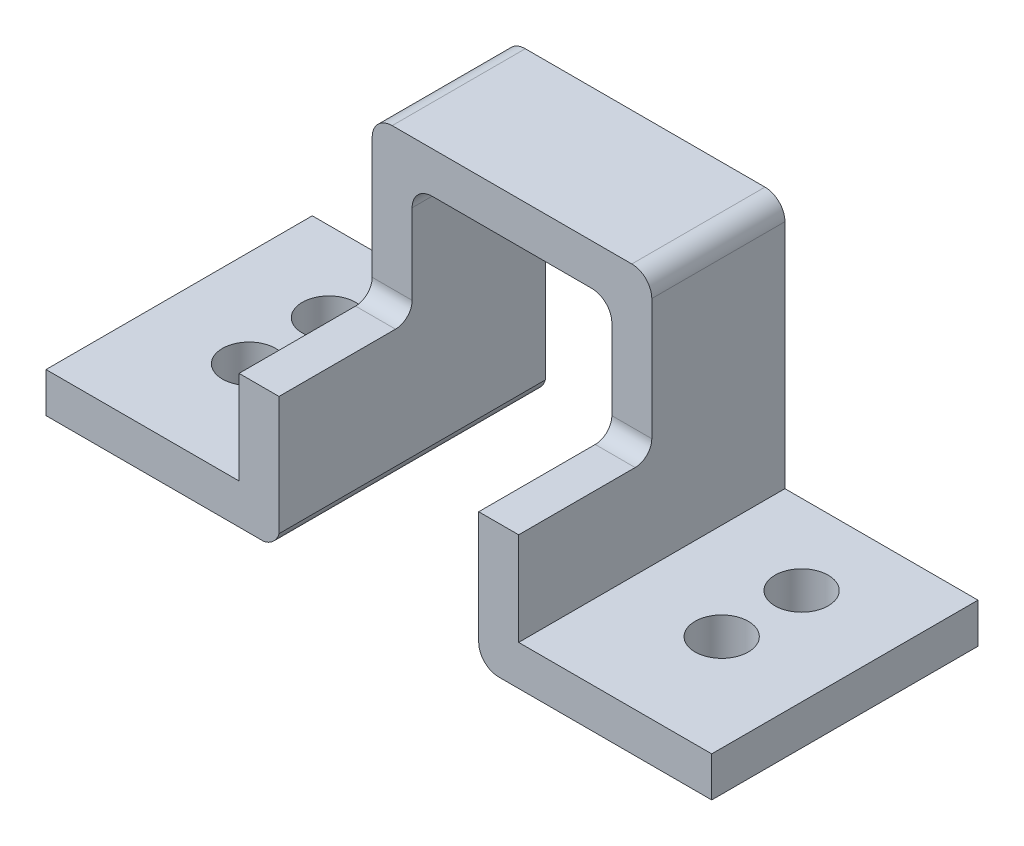
ISO-10303-21;
HEADER;
FILE_DESCRIPTION(('STEP AP214'),'2;1');
FILE_NAME('part.step','',(''),(''),'','','');
FILE_SCHEMA(('AUTOMOTIVE_DESIGN { 1 0 10303 214 1 1 1 1 }'));
ENDSEC;
DATA;
#1=APPLICATION_CONTEXT('core data for automotive mechanical design processes');
#2=APPLICATION_PROTOCOL_DEFINITION('international standard','automotive_design',2000,#1);
#3=PRODUCT_CONTEXT('',#1,'mechanical');
#4=PRODUCT('Part','Part','',(#3));
#5=PRODUCT_RELATED_PRODUCT_CATEGORY('part','',(#4));
#6=PRODUCT_DEFINITION_FORMATION('','',#4);
#7=PRODUCT_DEFINITION_CONTEXT('part definition',#1,'design');
#8=PRODUCT_DEFINITION('design','',#6,#7);
#9=PRODUCT_DEFINITION_SHAPE('','',#8);
#10=(LENGTH_UNIT() NAMED_UNIT(*) SI_UNIT(.MILLI.,.METRE.));
#11=(NAMED_UNIT(*) PLANE_ANGLE_UNIT() SI_UNIT($,.RADIAN.));
#12=(NAMED_UNIT(*) SI_UNIT($,.STERADIAN.) SOLID_ANGLE_UNIT());
#13=UNCERTAINTY_MEASURE_WITH_UNIT(LENGTH_MEASURE(1.E-05),#10,'distance_accuracy_value','');
#14=(GEOMETRIC_REPRESENTATION_CONTEXT(3) GLOBAL_UNCERTAINTY_ASSIGNED_CONTEXT((#13)) GLOBAL_UNIT_ASSIGNED_CONTEXT((#10,
#11,#12)) REPRESENTATION_CONTEXT('',''));
#15=CARTESIAN_POINT('',(0.,0.,0.));
#16=DIRECTION('',(0.,0.,1.));
#17=DIRECTION('',(1.,0.,0.));
#18=AXIS2_PLACEMENT_3D('',#15,#16,#17);
#19=CARTESIAN_POINT('',(0.,20.,28.));
#20=DIRECTION('',(0.,1.,0.));
#21=DIRECTION('',(0.,0.,1.));
#22=AXIS2_PLACEMENT_3D('',#19,#20,#21);
#23=PLANE('',#22);
#24=DIRECTION('',(0.,0.,-1.));
#25=VECTOR('',#24,1.);
#26=CARTESIAN_POINT('',(36.,20.,28.));
#27=LINE('',#26,#25);
#28=CARTESIAN_POINT('',(36.,20.,20.));
#29=VERTEX_POINT('',#28);
#30=CARTESIAN_POINT('',(36.,20.,2.49999999999997));
#31=VERTEX_POINT('',#30);
#32=EDGE_CURVE('E359',#29,#31,#27,.T.);
#33=ORIENTED_EDGE('',*,*,#32,.T.);
#34=DIRECTION('',(1.,0.,0.));
#35=VECTOR('',#34,1.);
#36=CARTESIAN_POINT('',(30.,20.,2.49999999999998));
#37=LINE('',#36,#35);
#38=CARTESIAN_POINT('',(30.,20.,2.49999999999997));
#39=VERTEX_POINT('',#38);
#40=EDGE_CURVE('E394',#39,#31,#37,.T.);
#41=ORIENTED_EDGE('',*,*,#40,.F.);
#42=DIRECTION('',(0.,0.,-1.));
#43=VECTOR('',#42,1.);
#44=CARTESIAN_POINT('',(30.,20.,28.));
#45=LINE('',#44,#43);
#46=CARTESIAN_POINT('',(30.,20.,20.));
#47=VERTEX_POINT('',#46);
#48=EDGE_CURVE('E323',#47,#39,#45,.T.);
#49=ORIENTED_EDGE('',*,*,#48,.F.);
#50=DIRECTION('',(-1.,0.,0.));
#51=VECTOR('',#50,1.);
#52=CARTESIAN_POINT('',(3.,20.,20.));
#53=LINE('',#52,#51);
#54=EDGE_CURVE('E50',#29,#47,#53,.T.);
#55=ORIENTED_EDGE('',*,*,#54,.F.);
#56=EDGE_LOOP('',(#33,#41,#49,#55));
#57=FACE_BOUND('',#56,.T.);
#58=ADVANCED_FACE('F39',(#57),#23,.T.);
#59=CARTESIAN_POINT('',(0.,0.,0.));
#60=DIRECTION('',(0.,0.,1.));
#61=DIRECTION('',(1.,0.,0.));
#62=AXIS2_PLACEMENT_3D('',#59,#60,#61);
#63=PLANE('',#62);
#64=DIRECTION('',(1.,0.,0.));
#65=VECTOR('',#64,1.);
#66=CARTESIAN_POINT('',(30.,22.5,0.));
#67=LINE('',#66,#65);
#68=CARTESIAN_POINT('',(30.,22.5,0.));
#69=VERTEX_POINT('',#68);
#70=CARTESIAN_POINT('',(36.,22.5,0.));
#71=VERTEX_POINT('',#70);
#72=EDGE_CURVE('E59',#69,#71,#67,.T.);
#73=ORIENTED_EDGE('',*,*,#72,.T.);
#74=DIRECTION('',(0.,1.,0.));
#75=VECTOR('',#74,1.);
#76=CARTESIAN_POINT('',(36.,0.,0.));
#77=LINE('',#76,#75);
#78=CARTESIAN_POINT('',(36.,40.7317104418747,0.));
#79=VERTEX_POINT('',#78);
#80=EDGE_CURVE('E358',#71,#79,#77,.T.);
#81=ORIENTED_EDGE('',*,*,#80,.T.);
#82=CARTESIAN_POINT('',(33.,40.7317104418747,0.));
#83=DIRECTION('',(0.,0.,1.));
#84=DIRECTION('',(1.,0.,0.));
#85=AXIS2_PLACEMENT_3D('',#82,#83,#84);
#86=CIRCLE('',#85,3.);
#87=CARTESIAN_POINT('',(33.,43.7317104418747,0.));
#88=VERTEX_POINT('',#87);
#89=EDGE_CURVE('E356',#79,#88,#86,.T.);
#90=ORIENTED_EDGE('',*,*,#89,.T.);
#91=DIRECTION('',(-1.,0.,0.));
#92=VECTOR('',#91,1.);
#93=CARTESIAN_POINT('',(0.,43.7317104418747,0.));
#94=LINE('',#93,#92);
#95=CARTESIAN_POINT('',(-3.,43.7317104418747,0.));
#96=VERTEX_POINT('',#95);
#97=EDGE_CURVE('E339',#88,#96,#94,.T.);
#98=ORIENTED_EDGE('',*,*,#97,.T.);
#99=CARTESIAN_POINT('',(-3.,40.7317104418747,0.));
#100=DIRECTION('',(0.,0.,1.));
#101=DIRECTION('',(1.,0.,0.));
#102=AXIS2_PLACEMENT_3D('',#99,#100,#101);
#103=CIRCLE('',#102,3.);
#104=CARTESIAN_POINT('',(-6.,40.7317104418747,0.));
#105=VERTEX_POINT('',#104);
#106=EDGE_CURVE('E344',#96,#105,#103,.T.);
#107=ORIENTED_EDGE('',*,*,#106,.T.);
#108=DIRECTION('',(0.,-1.,0.));
#109=VECTOR('',#108,1.);
#110=CARTESIAN_POINT('',(-5.99999999999999,0.,0.));
#111=LINE('',#110,#109);
#112=CARTESIAN_POINT('',(-6.,22.5,0.));
#113=VERTEX_POINT('',#112);
#114=EDGE_CURVE('E343',#105,#113,#111,.T.);
#115=ORIENTED_EDGE('',*,*,#114,.T.);
#116=DIRECTION('',(-1.,0.,0.));
#117=VECTOR('',#116,1.);
#118=CARTESIAN_POINT('',(0.,22.5,0.));
#119=LINE('',#118,#117);
#120=CARTESIAN_POINT('',(0.,22.5,0.));
#121=VERTEX_POINT('',#120);
#122=EDGE_CURVE('E219',#121,#113,#119,.T.);
#123=ORIENTED_EDGE('',*,*,#122,.F.);
#124=DIRECTION('',(0.,1.,0.));
#125=VECTOR('',#124,1.);
#126=CARTESIAN_POINT('',(0.,0.,0.));
#127=LINE('',#126,#125);
#128=CARTESIAN_POINT('',(0.,34.547795072297,0.));
#129=VERTEX_POINT('',#128);
#130=EDGE_CURVE('E349',#121,#129,#127,.T.);
#131=ORIENTED_EDGE('',*,*,#130,.T.);
#132=CARTESIAN_POINT('',(3.,34.547795072297,0.));
#133=DIRECTION('',(0.,0.,1.));
#134=DIRECTION('',(1.,0.,0.));
#135=AXIS2_PLACEMENT_3D('',#132,#133,#134);
#136=CIRCLE('',#135,3.);
#137=CARTESIAN_POINT('',(3.,37.547795072297,0.));
#138=VERTEX_POINT('',#137);
#139=EDGE_CURVE('E346',#129,#138,#136,.F.);
#140=ORIENTED_EDGE('',*,*,#139,.T.);
#141=DIRECTION('',(1.,0.,0.));
#142=VECTOR('',#141,1.);
#143=CARTESIAN_POINT('',(0.,37.547795072297,0.));
#144=LINE('',#143,#142);
#145=CARTESIAN_POINT('',(27.,37.547795072297,0.));
#146=VERTEX_POINT('',#145);
#147=EDGE_CURVE('E353',#138,#146,#144,.T.);
#148=ORIENTED_EDGE('',*,*,#147,.T.);
#149=CARTESIAN_POINT('',(27.,34.547795072297,0.));
#150=DIRECTION('',(0.,0.,1.));
#151=DIRECTION('',(1.,0.,0.));
#152=AXIS2_PLACEMENT_3D('',#149,#150,#151);
#153=CIRCLE('',#152,3.);
#154=CARTESIAN_POINT('',(30.,34.547795072297,0.));
#155=VERTEX_POINT('',#154);
#156=EDGE_CURVE('E351',#146,#155,#153,.F.);
#157=ORIENTED_EDGE('',*,*,#156,.T.);
#158=DIRECTION('',(0.,-1.,0.));
#159=VECTOR('',#158,1.);
#160=CARTESIAN_POINT('',(30.,0.,0.));
#161=LINE('',#160,#159);
#162=EDGE_CURVE('E53',#155,#69,#161,.T.);
#163=ORIENTED_EDGE('',*,*,#162,.T.);
#164=EDGE_LOOP('',(#73,#81,#90,#98,#107,#115,#123,#131,#140,#148,#157,#163));
#165=FACE_BOUND('',#164,.T.);
#166=ADVANCED_FACE('F426',(#165),#63,.T.);
#167=CARTESIAN_POINT('',(30.,34.547795072297,20.));
#168=DIRECTION('',(1.,0.,0.));
#169=DIRECTION('',(0.,1.,0.));
#170=AXIS2_PLACEMENT_3D('',#167,#168,#169);
#171=PLANE('',#170);
#172=CARTESIAN_POINT('',(30.,22.5,2.49999999999998));
#173=DIRECTION('',(-1.,0.,0.));
#174=DIRECTION('',(0.,0.,-1.));
#175=AXIS2_PLACEMENT_3D('',#172,#173,#174);
#176=CIRCLE('',#175,2.49999999999997);
#177=EDGE_CURVE('E440',#69,#39,#176,.T.);
#178=ORIENTED_EDGE('',*,*,#177,.F.);
#179=ORIENTED_EDGE('',*,*,#162,.F.);
#180=DIRECTION('',(0.,0.,-1.));
#181=VECTOR('',#180,1.);
#182=CARTESIAN_POINT('',(30.,34.547795072297,20.));
#183=LINE('',#182,#181);
#184=CARTESIAN_POINT('',(30.,34.547795072297,-20.));
#185=VERTEX_POINT('',#184);
#186=EDGE_CURVE('E309',#155,#185,#183,.T.);
#187=ORIENTED_EDGE('',*,*,#186,.T.);
#188=DIRECTION('',(0.,-1.,0.));
#189=VECTOR('',#188,1.);
#190=CARTESIAN_POINT('',(30.,34.547795072297,-20.));
#191=LINE('',#190,#189);
#192=CARTESIAN_POINT('',(30.,3.,-20.));
#193=VERTEX_POINT('',#192);
#194=EDGE_CURVE('E260',#185,#193,#191,.T.);
#195=ORIENTED_EDGE('',*,*,#194,.T.);
#196=DIRECTION('',(0.,0.,1.));
#197=VECTOR('',#196,1.);
#198=CARTESIAN_POINT('',(30.,3.,-20.));
#199=LINE('',#198,#197);
#200=CARTESIAN_POINT('',(30.,3.,20.));
#201=VERTEX_POINT('',#200);
#202=EDGE_CURVE('E210',#193,#201,#199,.T.);
#203=ORIENTED_EDGE('',*,*,#202,.T.);
#204=DIRECTION('',(0.,-1.,0.));
#205=VECTOR('',#204,1.);
#206=CARTESIAN_POINT('',(30.,34.547795072297,20.));
#207=LINE('',#206,#205);
#208=EDGE_CURVE('E217',#47,#201,#207,.T.);
#209=ORIENTED_EDGE('',*,*,#208,.F.);
#210=ORIENTED_EDGE('',*,*,#48,.T.);
#211=EDGE_LOOP('',(#178,#179,#187,#195,#203,#209,#210));
#212=FACE_BOUND('',#211,.T.);
#213=ADVANCED_FACE('F321',(#212),#171,.F.);
#214=CARTESIAN_POINT('',(3.,34.547795072297,20.));
#215=DIRECTION('',(0.,0.,1.));
#216=DIRECTION('',(1.,0.,0.));
#217=AXIS2_PLACEMENT_3D('',#214,#215,#216);
#218=PLANE('',#217);
#219=CARTESIAN_POINT('',(33.,3.,20.));
#220=DIRECTION('',(0.,0.,-1.));
#221=DIRECTION('',(1.,0.,0.));
#222=AXIS2_PLACEMENT_3D('',#219,#220,#221);
#223=CIRCLE('',#222,3.);
#224=CARTESIAN_POINT('',(33.,0.,20.));
#225=VERTEX_POINT('',#224);
#226=EDGE_CURVE('E198',#225,#201,#223,.T.);
#227=ORIENTED_EDGE('',*,*,#226,.F.);
#228=DIRECTION('',(1.,0.,0.));
#229=VECTOR('',#228,1.);
#230=CARTESIAN_POINT('',(30.,0.,20.));
#231=LINE('',#230,#229);
#232=CARTESIAN_POINT('',(65.,0.,20.));
#233=VERTEX_POINT('',#232);
#234=EDGE_CURVE('E215',#225,#233,#231,.T.);
#235=ORIENTED_EDGE('',*,*,#234,.T.);
#236=DIRECTION('',(0.,1.,0.));
#237=VECTOR('',#236,1.);
#238=CARTESIAN_POINT('',(65.,0.,20.));
#239=LINE('',#238,#237);
#240=CARTESIAN_POINT('',(65.,6.,20.));
#241=VERTEX_POINT('',#240);
#242=EDGE_CURVE('E221',#233,#241,#239,.T.);
#243=ORIENTED_EDGE('',*,*,#242,.T.);
#244=DIRECTION('',(-1.,0.,0.));
#245=VECTOR('',#244,1.);
#246=CARTESIAN_POINT('',(65.,6.,20.));
#247=LINE('',#246,#245);
#248=CARTESIAN_POINT('',(36.,6.,20.));
#249=VERTEX_POINT('',#248);
#250=EDGE_CURVE('E222',#241,#249,#247,.T.);
#251=ORIENTED_EDGE('',*,*,#250,.T.);
#252=DIRECTION('',(0.,1.,0.));
#253=VECTOR('',#252,1.);
#254=CARTESIAN_POINT('',(36.,6.,20.));
#255=LINE('',#254,#253);
#256=EDGE_CURVE('E235',#249,#29,#255,.T.);
#257=ORIENTED_EDGE('',*,*,#256,.T.);
#258=ORIENTED_EDGE('',*,*,#54,.T.);
#259=ORIENTED_EDGE('',*,*,#208,.T.);
#260=EDGE_LOOP('',(#227,#235,#243,#251,#257,#258,#259));
#261=FACE_BOUND('',#260,.T.);
#262=ADVANCED_FACE('F212',(#261),#218,.T.);
#263=CARTESIAN_POINT('',(3.,34.547795072297,-20.));
#264=DIRECTION('',(0.,0.,1.));
#265=DIRECTION('',(1.,0.,0.));
#266=AXIS2_PLACEMENT_3D('',#263,#264,#265);
#267=PLANE('',#266);
#268=DIRECTION('',(1.,0.,0.));
#269=VECTOR('',#268,1.);
#270=CARTESIAN_POINT('',(30.,0.,-20.));
#271=LINE('',#270,#269);
#272=CARTESIAN_POINT('',(33.,0.,-20.));
#273=VERTEX_POINT('',#272);
#274=CARTESIAN_POINT('',(65.,0.,-20.));
#275=VERTEX_POINT('',#274);
#276=EDGE_CURVE('E258',#273,#275,#271,.T.);
#277=ORIENTED_EDGE('',*,*,#276,.F.);
#278=CARTESIAN_POINT('',(33.,3.,-20.));
#279=DIRECTION('',(0.,0.,-1.));
#280=DIRECTION('',(1.,0.,0.));
#281=AXIS2_PLACEMENT_3D('',#278,#279,#280);
#282=CIRCLE('',#281,3.);
#283=EDGE_CURVE('E201',#273,#193,#282,.T.);
#284=ORIENTED_EDGE('',*,*,#283,.T.);
#285=ORIENTED_EDGE('',*,*,#194,.F.);
#286=CARTESIAN_POINT('',(27.,34.547795072297,-20.));
#287=DIRECTION('',(0.,0.,-1.));
#288=DIRECTION('',(1.,0.,0.));
#289=AXIS2_PLACEMENT_3D('',#286,#287,#288);
#290=CIRCLE('',#289,3.);
#291=CARTESIAN_POINT('',(27.,37.547795072297,-20.));
#292=VERTEX_POINT('',#291);
#293=EDGE_CURVE('E251',#292,#185,#290,.T.);
#294=ORIENTED_EDGE('',*,*,#293,.F.);
#295=DIRECTION('',(1.,0.,0.));
#296=VECTOR('',#295,1.);
#297=CARTESIAN_POINT('',(3.,37.547795072297,-20.));
#298=LINE('',#297,#296);
#299=CARTESIAN_POINT('',(3.,37.547795072297,-20.));
#300=VERTEX_POINT('',#299);
#301=EDGE_CURVE('E252',#300,#292,#298,.T.);
#302=ORIENTED_EDGE('',*,*,#301,.F.);
#303=CARTESIAN_POINT('',(3.,34.547795072297,-20.));
#304=DIRECTION('',(0.,0.,-1.));
#305=DIRECTION('',(1.,0.,0.));
#306=AXIS2_PLACEMENT_3D('',#303,#304,#305);
#307=CIRCLE('',#306,3.);
#308=CARTESIAN_POINT('',(0.,34.547795072297,-20.));
#309=VERTEX_POINT('',#308);
#310=EDGE_CURVE('E250',#309,#300,#307,.T.);
#311=ORIENTED_EDGE('',*,*,#310,.F.);
#312=DIRECTION('',(0.,1.,0.));
#313=VECTOR('',#312,1.);
#314=CARTESIAN_POINT('',(0.,0.,-20.));
#315=LINE('',#314,#313);
#316=CARTESIAN_POINT('',(0.,2.14044011670868,-20.));
#317=VERTEX_POINT('',#316);
#318=EDGE_CURVE('E244',#317,#309,#315,.T.);
#319=ORIENTED_EDGE('',*,*,#318,.F.);
#320=CARTESIAN_POINT('',(-2.89404902944698,2.93068072257311,-20.));
#321=DIRECTION('',(0.,0.,-1.));
#322=DIRECTION('',(-1.,0.,0.));
#323=AXIS2_PLACEMENT_3D('',#320,#321,#322);
#324=CIRCLE('',#323,3.);
#325=CARTESIAN_POINT('',(-2.25287003545363,0.,-20.));
#326=VERTEX_POINT('',#325);
#327=EDGE_CURVE('E328',#317,#326,#324,.T.);
#328=ORIENTED_EDGE('',*,*,#327,.T.);
#329=DIRECTION('',(1.,0.,0.));
#330=VECTOR('',#329,1.);
#331=CARTESIAN_POINT('',(-35.,0.,-20.));
#332=LINE('',#331,#330);
#333=CARTESIAN_POINT('',(-35.,0.,-20.));
#334=VERTEX_POINT('',#333);
#335=EDGE_CURVE('E281',#334,#326,#332,.T.);
#336=ORIENTED_EDGE('',*,*,#335,.F.);
#337=DIRECTION('',(0.,-1.,0.));
#338=VECTOR('',#337,1.);
#339=CARTESIAN_POINT('',(-35.,6.,-20.));
#340=LINE('',#339,#338);
#341=CARTESIAN_POINT('',(-35.,6.,-20.));
#342=VERTEX_POINT('',#341);
#343=EDGE_CURVE('E284',#342,#334,#340,.T.);
#344=ORIENTED_EDGE('',*,*,#343,.F.);
#345=DIRECTION('',(-1.,0.,0.));
#346=VECTOR('',#345,1.);
#347=CARTESIAN_POINT('',(-6.,6.,-20.));
#348=LINE('',#347,#346);
#349=CARTESIAN_POINT('',(-6.,6.,-20.));
#350=VERTEX_POINT('',#349);
#351=EDGE_CURVE('E278',#350,#342,#348,.T.);
#352=ORIENTED_EDGE('',*,*,#351,.F.);
#353=DIRECTION('',(0.,-1.,0.));
#354=VECTOR('',#353,1.);
#355=CARTESIAN_POINT('',(-6.,40.7317104418747,-20.));
#356=LINE('',#355,#354);
#357=CARTESIAN_POINT('',(-6.,40.7317104418747,-20.));
#358=VERTEX_POINT('',#357);
#359=EDGE_CURVE('E279',#358,#350,#356,.T.);
#360=ORIENTED_EDGE('',*,*,#359,.F.);
#361=CARTESIAN_POINT('',(-3.,40.7317104418747,-20.));
#362=DIRECTION('',(0.,0.,1.));
#363=DIRECTION('',(1.,0.,0.));
#364=AXIS2_PLACEMENT_3D('',#361,#362,#363);
#365=CIRCLE('',#364,3.);
#366=CARTESIAN_POINT('',(-3.,43.7317104418747,-20.));
#367=VERTEX_POINT('',#366);
#368=EDGE_CURVE('E273',#367,#358,#365,.T.);
#369=ORIENTED_EDGE('',*,*,#368,.F.);
#370=DIRECTION('',(-1.,0.,0.));
#371=VECTOR('',#370,1.);
#372=CARTESIAN_POINT('',(33.,43.7317104418747,-20.));
#373=LINE('',#372,#371);
#374=CARTESIAN_POINT('',(33.,43.7317104418747,-20.));
#375=VERTEX_POINT('',#374);
#376=EDGE_CURVE('E275',#375,#367,#373,.T.);
#377=ORIENTED_EDGE('',*,*,#376,.F.);
#378=CARTESIAN_POINT('',(33.,40.7317104418747,-20.));
#379=DIRECTION('',(0.,0.,1.));
#380=DIRECTION('',(1.,0.,0.));
#381=AXIS2_PLACEMENT_3D('',#378,#379,#380);
#382=CIRCLE('',#381,3.);
#383=CARTESIAN_POINT('',(36.,40.7317104418747,-20.));
#384=VERTEX_POINT('',#383);
#385=EDGE_CURVE('E269',#384,#375,#382,.T.);
#386=ORIENTED_EDGE('',*,*,#385,.F.);
#387=DIRECTION('',(0.,1.,0.));
#388=VECTOR('',#387,1.);
#389=CARTESIAN_POINT('',(36.,6.,-20.));
#390=LINE('',#389,#388);
#391=CARTESIAN_POINT('',(36.,6.,-20.));
#392=VERTEX_POINT('',#391);
#393=EDGE_CURVE('E268',#392,#384,#390,.T.);
#394=ORIENTED_EDGE('',*,*,#393,.F.);
#395=DIRECTION('',(-1.,0.,0.));
#396=VECTOR('',#395,1.);
#397=CARTESIAN_POINT('',(65.,6.,-20.));
#398=LINE('',#397,#396);
#399=CARTESIAN_POINT('',(65.,6.,-20.));
#400=VERTEX_POINT('',#399);
#401=EDGE_CURVE('E261',#400,#392,#398,.T.);
#402=ORIENTED_EDGE('',*,*,#401,.F.);
#403=DIRECTION('',(0.,1.,0.));
#404=VECTOR('',#403,1.);
#405=CARTESIAN_POINT('',(65.,0.,-20.));
#406=LINE('',#405,#404);
#407=EDGE_CURVE('E264',#275,#400,#406,.T.);
#408=ORIENTED_EDGE('',*,*,#407,.F.);
#409=EDGE_LOOP('',(#277,#284,#285,#294,#302,#311,#319,#328,#336,#344,#352,#360,#369,#377,#386,
#394,#402,#408));
#410=FACE_BOUND('',#409,.T.);
#411=ADVANCED_FACE('F417',(#410),#267,.F.);
#412=CARTESIAN_POINT('',(0.,0.,20.));
#413=DIRECTION('',(-1.,0.,0.));
#414=DIRECTION('',(0.,0.,1.));
#415=AXIS2_PLACEMENT_3D('',#412,#413,#414);
#416=PLANE('',#415);
#417=CARTESIAN_POINT('',(0.,22.5,2.5));
#418=DIRECTION('',(1.,0.,0.));
#419=DIRECTION('',(0.,-1.,0.));
#420=AXIS2_PLACEMENT_3D('',#417,#418,#419);
#421=CIRCLE('',#420,2.5);
#422=CARTESIAN_POINT('',(0.,20.,2.5));
#423=VERTEX_POINT('',#422);
#424=EDGE_CURVE('E382',#423,#121,#421,.T.);
#425=ORIENTED_EDGE('',*,*,#424,.F.);
#426=DIRECTION('',(0.,0.,-1.));
#427=VECTOR('',#426,1.);
#428=CARTESIAN_POINT('',(0.,20.,28.));
#429=LINE('',#428,#427);
#430=CARTESIAN_POINT('',(0.,20.,20.));
#431=VERTEX_POINT('',#430);
#432=EDGE_CURVE('E361',#431,#423,#429,.T.);
#433=ORIENTED_EDGE('',*,*,#432,.F.);
#434=DIRECTION('',(0.,1.,0.));
#435=VECTOR('',#434,1.);
#436=CARTESIAN_POINT('',(0.,0.,20.));
#437=LINE('',#436,#435);
#438=CARTESIAN_POINT('',(0.,2.14044011670868,20.));
#439=VERTEX_POINT('',#438);
#440=EDGE_CURVE('E227',#439,#431,#437,.T.);
#441=ORIENTED_EDGE('',*,*,#440,.F.);
#442=DIRECTION('',(0.,0.,1.));
#443=VECTOR('',#442,1.);
#444=CARTESIAN_POINT('',(0.,2.14044011670868,-20.));
#445=LINE('',#444,#443);
#446=EDGE_CURVE('E340',#317,#439,#445,.T.);
#447=ORIENTED_EDGE('',*,*,#446,.F.);
#448=ORIENTED_EDGE('',*,*,#318,.T.);
#449=DIRECTION('',(0.,0.,-1.));
#450=VECTOR('',#449,1.);
#451=CARTESIAN_POINT('',(0.,34.547795072297,20.));
#452=LINE('',#451,#450);
#453=EDGE_CURVE('E317',#129,#309,#452,.T.);
#454=ORIENTED_EDGE('',*,*,#453,.F.);
#455=ORIENTED_EDGE('',*,*,#130,.F.);
#456=EDGE_LOOP('',(#425,#433,#441,#447,#448,#454,#455));
#457=FACE_BOUND('',#456,.T.);
#458=ADVANCED_FACE('F41',(#457),#416,.F.);
#459=CARTESIAN_POINT('',(3.,34.547795072297,20.));
#460=DIRECTION('',(0.,0.,-1.));
#461=DIRECTION('',(-1.,0.,0.));
#462=AXIS2_PLACEMENT_3D('',#459,#460,#461);
#463=CYLINDRICAL_SURFACE('',#462,3.);
#464=ORIENTED_EDGE('',*,*,#139,.F.);
#465=ORIENTED_EDGE('',*,*,#453,.T.);
#466=ORIENTED_EDGE('',*,*,#310,.T.);
#467=DIRECTION('',(0.,0.,-1.));
#468=VECTOR('',#467,1.);
#469=CARTESIAN_POINT('',(3.,37.547795072297,20.));
#470=LINE('',#469,#468);
#471=EDGE_CURVE('E313',#138,#300,#470,.T.);
#472=ORIENTED_EDGE('',*,*,#471,.F.);
#473=EDGE_LOOP('',(#464,#465,#466,#472));
#474=FACE_BOUND('',#473,.T.);
#475=ADVANCED_FACE('F424',(#474),#463,.F.);
#476=CARTESIAN_POINT('',(3.,37.547795072297,20.));
#477=DIRECTION('',(0.,1.,0.));
#478=DIRECTION('',(0.,0.,1.));
#479=AXIS2_PLACEMENT_3D('',#476,#477,#478);
#480=PLANE('',#479);
#481=ORIENTED_EDGE('',*,*,#147,.F.);
#482=ORIENTED_EDGE('',*,*,#471,.T.);
#483=ORIENTED_EDGE('',*,*,#301,.T.);
#484=DIRECTION('',(0.,0.,-1.));
#485=VECTOR('',#484,1.);
#486=CARTESIAN_POINT('',(27.,37.547795072297,20.));
#487=LINE('',#486,#485);
#488=EDGE_CURVE('E315',#146,#292,#487,.T.);
#489=ORIENTED_EDGE('',*,*,#488,.F.);
#490=EDGE_LOOP('',(#481,#482,#483,#489));
#491=FACE_BOUND('',#490,.T.);
#492=ADVANCED_FACE('F435',(#491),#480,.F.);
#493=CARTESIAN_POINT('',(27.,34.547795072297,20.));
#494=DIRECTION('',(0.,0.,-1.));
#495=DIRECTION('',(-1.,0.,0.));
#496=AXIS2_PLACEMENT_3D('',#493,#494,#495);
#497=CYLINDRICAL_SURFACE('',#496,3.);
#498=ORIENTED_EDGE('',*,*,#156,.F.);
#499=ORIENTED_EDGE('',*,*,#488,.T.);
#500=ORIENTED_EDGE('',*,*,#293,.T.);
#501=ORIENTED_EDGE('',*,*,#186,.F.);
#502=EDGE_LOOP('',(#498,#499,#500,#501));
#503=FACE_BOUND('',#502,.T.);
#504=ADVANCED_FACE('F434',(#503),#497,.F.);
#505=CARTESIAN_POINT('',(36.,6.,20.));
#506=DIRECTION('',(-1.,0.,0.));
#507=DIRECTION('',(0.,0.,1.));
#508=AXIS2_PLACEMENT_3D('',#505,#506,#507);
#509=PLANE('',#508);
#510=ORIENTED_EDGE('',*,*,#80,.F.);
#511=CARTESIAN_POINT('',(36.,22.5,2.49999999999998));
#512=DIRECTION('',(-1.,0.,0.));
#513=DIRECTION('',(0.,0.,-1.));
#514=AXIS2_PLACEMENT_3D('',#511,#512,#513);
#515=CIRCLE('',#514,2.49999999999997);
#516=EDGE_CURVE('E439',#71,#31,#515,.T.);
#517=ORIENTED_EDGE('',*,*,#516,.T.);
#518=ORIENTED_EDGE('',*,*,#32,.F.);
#519=ORIENTED_EDGE('',*,*,#256,.F.);
#520=DIRECTION('',(0.,0.,-1.));
#521=VECTOR('',#520,1.);
#522=CARTESIAN_POINT('',(36.,6.,20.));
#523=LINE('',#522,#521);
#524=EDGE_CURVE('E303',#249,#392,#523,.T.);
#525=ORIENTED_EDGE('',*,*,#524,.T.);
#526=ORIENTED_EDGE('',*,*,#393,.T.);
#527=DIRECTION('',(0.,0.,-1.));
#528=VECTOR('',#527,1.);
#529=CARTESIAN_POINT('',(36.,40.7317104418747,20.));
#530=LINE('',#529,#528);
#531=EDGE_CURVE('E301',#79,#384,#530,.T.);
#532=ORIENTED_EDGE('',*,*,#531,.F.);
#533=EDGE_LOOP('',(#510,#517,#518,#519,#525,#526,#532));
#534=FACE_BOUND('',#533,.T.);
#535=ADVANCED_FACE('F596',(#534),#509,.F.);
#536=CARTESIAN_POINT('',(33.,40.7317104418747,20.));
#537=DIRECTION('',(0.,0.,-1.));
#538=DIRECTION('',(-1.,0.,0.));
#539=AXIS2_PLACEMENT_3D('',#536,#537,#538);
#540=CYLINDRICAL_SURFACE('',#539,3.);
#541=ORIENTED_EDGE('',*,*,#89,.F.);
#542=ORIENTED_EDGE('',*,*,#531,.T.);
#543=ORIENTED_EDGE('',*,*,#385,.T.);
#544=DIRECTION('',(0.,0.,-1.));
#545=VECTOR('',#544,1.);
#546=CARTESIAN_POINT('',(33.,43.7317104418747,20.));
#547=LINE('',#546,#545);
#548=EDGE_CURVE('E299',#88,#375,#547,.T.);
#549=ORIENTED_EDGE('',*,*,#548,.F.);
#550=EDGE_LOOP('',(#541,#542,#543,#549));
#551=FACE_BOUND('',#550,.T.);
#552=ADVANCED_FACE('F604',(#551),#540,.T.);
#553=CARTESIAN_POINT('',(33.,43.7317104418747,20.));
#554=DIRECTION('',(0.,-1.,0.));
#555=DIRECTION('',(0.,0.,-1.));
#556=AXIS2_PLACEMENT_3D('',#553,#554,#555);
#557=PLANE('',#556);
#558=ORIENTED_EDGE('',*,*,#97,.F.);
#559=ORIENTED_EDGE('',*,*,#548,.T.);
#560=ORIENTED_EDGE('',*,*,#376,.T.);
#561=DIRECTION('',(0.,0.,-1.));
#562=VECTOR('',#561,1.);
#563=CARTESIAN_POINT('',(-3.,43.7317104418747,20.));
#564=LINE('',#563,#562);
#565=EDGE_CURVE('E300',#96,#367,#564,.T.);
#566=ORIENTED_EDGE('',*,*,#565,.F.);
#567=EDGE_LOOP('',(#558,#559,#560,#566));
#568=FACE_BOUND('',#567,.T.);
#569=ADVANCED_FACE('F664',(#568),#557,.F.);
#570=CARTESIAN_POINT('',(-3.,40.7317104418747,20.));
#571=DIRECTION('',(0.,0.,-1.));
#572=DIRECTION('',(-1.,0.,0.));
#573=AXIS2_PLACEMENT_3D('',#570,#571,#572);
#574=CYLINDRICAL_SURFACE('',#573,3.);
#575=ORIENTED_EDGE('',*,*,#106,.F.);
#576=ORIENTED_EDGE('',*,*,#565,.T.);
#577=ORIENTED_EDGE('',*,*,#368,.T.);
#578=DIRECTION('',(0.,0.,-1.));
#579=VECTOR('',#578,1.);
#580=CARTESIAN_POINT('',(-6.,40.7317104418747,20.));
#581=LINE('',#580,#579);
#582=EDGE_CURVE('E294',#105,#358,#581,.T.);
#583=ORIENTED_EDGE('',*,*,#582,.F.);
#584=EDGE_LOOP('',(#575,#576,#577,#583));
#585=FACE_BOUND('',#584,.T.);
#586=ADVANCED_FACE('F566',(#585),#574,.T.);
#587=CARTESIAN_POINT('',(-6.,40.7317104418747,20.));
#588=DIRECTION('',(1.,0.,0.));
#589=DIRECTION('',(0.,1.,0.));
#590=AXIS2_PLACEMENT_3D('',#587,#588,#589);
#591=PLANE('',#590);
#592=DIRECTION('',(0.,0.,-1.));
#593=VECTOR('',#592,1.);
#594=CARTESIAN_POINT('',(-6.,20.,28.));
#595=LINE('',#594,#593);
#596=CARTESIAN_POINT('',(-6.,20.,20.));
#597=VERTEX_POINT('',#596);
#598=CARTESIAN_POINT('',(-6.,20.,2.5));
#599=VERTEX_POINT('',#598);
#600=EDGE_CURVE('E247',#597,#599,#595,.T.);
#601=ORIENTED_EDGE('',*,*,#600,.T.);
#602=CARTESIAN_POINT('',(-6.,22.5,2.5));
#603=DIRECTION('',(1.,0.,0.));
#604=DIRECTION('',(0.,-1.,0.));
#605=AXIS2_PLACEMENT_3D('',#602,#603,#604);
#606=CIRCLE('',#605,2.5);
#607=EDGE_CURVE('E387',#599,#113,#606,.T.);
#608=ORIENTED_EDGE('',*,*,#607,.T.);
#609=ORIENTED_EDGE('',*,*,#114,.F.);
#610=ORIENTED_EDGE('',*,*,#582,.T.);
#611=ORIENTED_EDGE('',*,*,#359,.T.);
#612=DIRECTION('',(0.,0.,-1.));
#613=VECTOR('',#612,1.);
#614=CARTESIAN_POINT('',(-6.,6.,20.));
#615=LINE('',#614,#613);
#616=CARTESIAN_POINT('',(-6.,6.,20.));
#617=VERTEX_POINT('',#616);
#618=EDGE_CURVE('E292',#617,#350,#615,.T.);
#619=ORIENTED_EDGE('',*,*,#618,.F.);
#620=DIRECTION('',(0.,-1.,0.));
#621=VECTOR('',#620,1.);
#622=CARTESIAN_POINT('',(-6.,40.7317104418747,20.));
#623=LINE('',#622,#621);
#624=EDGE_CURVE('E232',#597,#617,#623,.T.);
#625=ORIENTED_EDGE('',*,*,#624,.F.);
#626=EDGE_LOOP('',(#601,#608,#609,#610,#611,#619,#625));
#627=FACE_BOUND('',#626,.T.);
#628=ADVANCED_FACE('F399',(#627),#591,.F.);
#629=CARTESIAN_POINT('',(-2.89404902944698,2.93068072257311,20.));
#630=DIRECTION('',(0.,0.,-1.));
#631=DIRECTION('',(-1.,0.,0.));
#632=AXIS2_PLACEMENT_3D('',#629,#630,#631);
#633=CIRCLE('',#632,3.);
#634=CARTESIAN_POINT('',(-2.25287003545363,0.,20.));
#635=VERTEX_POINT('',#634);
#636=EDGE_CURVE('E330',#439,#635,#633,.T.);
#637=ORIENTED_EDGE('',*,*,#636,.F.);
#638=ORIENTED_EDGE('',*,*,#440,.T.);
#639=DIRECTION('',(-1.,0.,0.));
#640=VECTOR('',#639,1.);
#641=CARTESIAN_POINT('',(3.,20.,20.));
#642=LINE('',#641,#640);
#643=EDGE_CURVE('E11',#431,#597,#642,.T.);
#644=ORIENTED_EDGE('',*,*,#643,.T.);
#645=ORIENTED_EDGE('',*,*,#624,.T.);
#646=DIRECTION('',(-1.,0.,0.));
#647=VECTOR('',#646,1.);
#648=CARTESIAN_POINT('',(-6.,6.,20.));
#649=LINE('',#648,#647);
#650=CARTESIAN_POINT('',(-35.,6.,20.));
#651=VERTEX_POINT('',#650);
#652=EDGE_CURVE('E240',#617,#651,#649,.T.);
#653=ORIENTED_EDGE('',*,*,#652,.T.);
#654=DIRECTION('',(0.,-1.,0.));
#655=VECTOR('',#654,1.);
#656=CARTESIAN_POINT('',(-35.,6.,20.));
#657=LINE('',#656,#655);
#658=CARTESIAN_POINT('',(-35.,0.,20.));
#659=VERTEX_POINT('',#658);
#660=EDGE_CURVE('E237',#651,#659,#657,.T.);
#661=ORIENTED_EDGE('',*,*,#660,.T.);
#662=DIRECTION('',(1.,0.,0.));
#663=VECTOR('',#662,1.);
#664=CARTESIAN_POINT('',(-35.,0.,20.));
#665=LINE('',#664,#663);
#666=EDGE_CURVE('E241',#659,#635,#665,.T.);
#667=ORIENTED_EDGE('',*,*,#666,.T.);
#668=EDGE_LOOP('',(#637,#638,#644,#645,#653,#661,#667));
#669=FACE_BOUND('',#668,.T.);
#670=ADVANCED_FACE('F369',(#669),#218,.T.);
#671=CARTESIAN_POINT('',(30.,0.,20.));
#672=DIRECTION('',(0.,1.,0.));
#673=DIRECTION('',(0.,0.,1.));
#674=AXIS2_PLACEMENT_3D('',#671,#672,#673);
#675=PLANE('',#674);
#676=CARTESIAN_POINT('',(50.5,0.,-8.));
#677=DIRECTION('',(0.,1.,0.));
#678=DIRECTION('',(-1.,0.,0.));
#679=AXIS2_PLACEMENT_3D('',#676,#677,#678);
#680=CIRCLE('',#679,4.00000000000001);
#681=CARTESIAN_POINT('',(46.5,0.,-8.));
#682=VERTEX_POINT('',#681);
#683=EDGE_CURVE('E446',#682,#682,#680,.T.);
#684=ORIENTED_EDGE('',*,*,#683,.T.);
#685=EDGE_LOOP('',(#684));
#686=FACE_BOUND('',#685,.T.);
#687=CARTESIAN_POINT('',(50.5,0.,4.));
#688=DIRECTION('',(0.,1.,0.));
#689=DIRECTION('',(-1.,0.,0.));
#690=AXIS2_PLACEMENT_3D('',#687,#688,#689);
#691=CIRCLE('',#690,4.00000000000001);
#692=CARTESIAN_POINT('',(46.5,0.,4.));
#693=VERTEX_POINT('',#692);
#694=EDGE_CURVE('E442',#693,#693,#691,.T.);
#695=ORIENTED_EDGE('',*,*,#694,.T.);
#696=EDGE_LOOP('',(#695));
#697=FACE_BOUND('',#696,.T.);
#698=ORIENTED_EDGE('',*,*,#234,.F.);
#699=DIRECTION('',(0.,0.,1.));
#700=VECTOR('',#699,1.);
#701=CARTESIAN_POINT('',(33.,0.,-20.));
#702=LINE('',#701,#700);
#703=EDGE_CURVE('E199',#273,#225,#702,.T.);
#704=ORIENTED_EDGE('',*,*,#703,.F.);
#705=ORIENTED_EDGE('',*,*,#276,.T.);
#706=DIRECTION('',(0.,0.,-1.));
#707=VECTOR('',#706,1.);
#708=CARTESIAN_POINT('',(65.,0.,20.));
#709=LINE('',#708,#707);
#710=EDGE_CURVE('E223',#233,#275,#709,.T.);
#711=ORIENTED_EDGE('',*,*,#710,.F.);
#712=EDGE_LOOP('',(#698,#704,#705,#711));
#713=FACE_BOUND('',#712,.T.);
#714=ADVANCED_FACE('F216',(#686,#697,#713),#675,.F.);
#715=CARTESIAN_POINT('',(65.,0.,20.));
#716=DIRECTION('',(-1.,0.,0.));
#717=DIRECTION('',(0.,0.,1.));
#718=AXIS2_PLACEMENT_3D('',#715,#716,#717);
#719=PLANE('',#718);
#720=ORIENTED_EDGE('',*,*,#407,.T.);
#721=DIRECTION('',(0.,0.,-1.));
#722=VECTOR('',#721,1.);
#723=CARTESIAN_POINT('',(65.,6.,20.));
#724=LINE('',#723,#722);
#725=EDGE_CURVE('E306',#241,#400,#724,.T.);
#726=ORIENTED_EDGE('',*,*,#725,.F.);
#727=ORIENTED_EDGE('',*,*,#242,.F.);
#728=ORIENTED_EDGE('',*,*,#710,.T.);
#729=EDGE_LOOP('',(#720,#726,#727,#728));
#730=FACE_BOUND('',#729,.T.);
#731=ADVANCED_FACE('F490',(#730),#719,.F.);
#732=CARTESIAN_POINT('',(65.,6.,20.));
#733=DIRECTION('',(0.,-1.,0.));
#734=DIRECTION('',(1.,0.,0.));
#735=AXIS2_PLACEMENT_3D('',#732,#733,#734);
#736=PLANE('',#735);
#737=CARTESIAN_POINT('',(50.5,6.,-8.));
#738=DIRECTION('',(0.,1.,0.));
#739=DIRECTION('',(-1.,0.,0.));
#740=AXIS2_PLACEMENT_3D('',#737,#738,#739);
#741=CIRCLE('',#740,4.00000000000001);
#742=CARTESIAN_POINT('',(46.5,6.,-8.));
#743=VERTEX_POINT('',#742);
#744=EDGE_CURVE('E456',#743,#743,#741,.T.);
#745=ORIENTED_EDGE('',*,*,#744,.F.);
#746=EDGE_LOOP('',(#745));
#747=FACE_BOUND('',#746,.T.);
#748=CARTESIAN_POINT('',(50.5,6.,4.));
#749=DIRECTION('',(0.,1.,0.));
#750=DIRECTION('',(-1.,0.,0.));
#751=AXIS2_PLACEMENT_3D('',#748,#749,#750);
#752=CIRCLE('',#751,4.00000000000001);
#753=CARTESIAN_POINT('',(46.5,6.,4.));
#754=VERTEX_POINT('',#753);
#755=EDGE_CURVE('E447',#754,#754,#752,.T.);
#756=ORIENTED_EDGE('',*,*,#755,.F.);
#757=EDGE_LOOP('',(#756));
#758=FACE_BOUND('',#757,.T.);
#759=ORIENTED_EDGE('',*,*,#401,.T.);
#760=ORIENTED_EDGE('',*,*,#524,.F.);
#761=ORIENTED_EDGE('',*,*,#250,.F.);
#762=ORIENTED_EDGE('',*,*,#725,.T.);
#763=EDGE_LOOP('',(#759,#760,#761,#762));
#764=FACE_BOUND('',#763,.T.);
#765=ADVANCED_FACE('F478',(#747,#758,#764),#736,.F.);
#766=CARTESIAN_POINT('',(-6.,6.,20.));
#767=DIRECTION('',(0.,-1.,0.));
#768=DIRECTION('',(1.,0.,0.));
#769=AXIS2_PLACEMENT_3D('',#766,#767,#768);
#770=PLANE('',#769);
#771=CARTESIAN_POINT('',(-20.5,5.99999999999999,4.));
#772=DIRECTION('',(0.,1.,0.));
#773=DIRECTION('',(1.,0.,0.));
#774=AXIS2_PLACEMENT_3D('',#771,#772,#773);
#775=CIRCLE('',#774,4.00000000000001);
#776=CARTESIAN_POINT('',(-16.5,5.99999999999999,4.));
#777=VERTEX_POINT('',#776);
#778=EDGE_CURVE('E455',#777,#777,#775,.T.);
#779=ORIENTED_EDGE('',*,*,#778,.F.);
#780=EDGE_LOOP('',(#779));
#781=FACE_BOUND('',#780,.T.);
#782=CARTESIAN_POINT('',(-20.5,5.99999999999999,-8.));
#783=DIRECTION('',(0.,1.,0.));
#784=DIRECTION('',(1.,0.,0.));
#785=AXIS2_PLACEMENT_3D('',#782,#783,#784);
#786=CIRCLE('',#785,4.00000000000001);
#787=CARTESIAN_POINT('',(-16.5,5.99999999999999,-8.));
#788=VERTEX_POINT('',#787);
#789=EDGE_CURVE('E464',#788,#788,#786,.T.);
#790=ORIENTED_EDGE('',*,*,#789,.F.);
#791=EDGE_LOOP('',(#790));
#792=FACE_BOUND('',#791,.T.);
#793=ORIENTED_EDGE('',*,*,#351,.T.);
#794=DIRECTION('',(0.,0.,-1.));
#795=VECTOR('',#794,1.);
#796=CARTESIAN_POINT('',(-35.,6.,20.));
#797=LINE('',#796,#795);
#798=EDGE_CURVE('E289',#651,#342,#797,.T.);
#799=ORIENTED_EDGE('',*,*,#798,.F.);
#800=ORIENTED_EDGE('',*,*,#652,.F.);
#801=ORIENTED_EDGE('',*,*,#618,.T.);
#802=EDGE_LOOP('',(#793,#799,#800,#801));
#803=FACE_BOUND('',#802,.T.);
#804=ADVANCED_FACE('F410',(#781,#792,#803),#770,.F.);
#805=CARTESIAN_POINT('',(-35.,6.,20.));
#806=DIRECTION('',(1.,0.,0.));
#807=DIRECTION('',(0.,0.,-1.));
#808=AXIS2_PLACEMENT_3D('',#805,#806,#807);
#809=PLANE('',#808);
#810=ORIENTED_EDGE('',*,*,#343,.T.);
#811=DIRECTION('',(0.,0.,-1.));
#812=VECTOR('',#811,1.);
#813=CARTESIAN_POINT('',(-35.,0.,20.));
#814=LINE('',#813,#812);
#815=EDGE_CURVE('E242',#659,#334,#814,.T.);
#816=ORIENTED_EDGE('',*,*,#815,.F.);
#817=ORIENTED_EDGE('',*,*,#660,.F.);
#818=ORIENTED_EDGE('',*,*,#798,.T.);
#819=EDGE_LOOP('',(#810,#816,#817,#818));
#820=FACE_BOUND('',#819,.T.);
#821=ADVANCED_FACE('F412',(#820),#809,.F.);
#822=CARTESIAN_POINT('',(-35.,0.,20.));
#823=DIRECTION('',(0.,1.,0.));
#824=DIRECTION('',(0.,0.,1.));
#825=AXIS2_PLACEMENT_3D('',#822,#823,#824);
#826=PLANE('',#825);
#827=CARTESIAN_POINT('',(-20.5,0.,4.));
#828=DIRECTION('',(0.,1.,0.));
#829=DIRECTION('',(1.,0.,0.));
#830=AXIS2_PLACEMENT_3D('',#827,#828,#829);
#831=CIRCLE('',#830,4.00000000000001);
#832=CARTESIAN_POINT('',(-16.5,0.,4.));
#833=VERTEX_POINT('',#832);
#834=EDGE_CURVE('E453',#833,#833,#831,.T.);
#835=ORIENTED_EDGE('',*,*,#834,.T.);
#836=EDGE_LOOP('',(#835));
#837=FACE_BOUND('',#836,.T.);
#838=CARTESIAN_POINT('',(-20.5,0.,-8.));
#839=DIRECTION('',(0.,1.,0.));
#840=DIRECTION('',(1.,0.,0.));
#841=AXIS2_PLACEMENT_3D('',#838,#839,#840);
#842=CIRCLE('',#841,4.00000000000001);
#843=CARTESIAN_POINT('',(-16.5,0.,-8.));
#844=VERTEX_POINT('',#843);
#845=EDGE_CURVE('E457',#844,#844,#842,.T.);
#846=ORIENTED_EDGE('',*,*,#845,.T.);
#847=EDGE_LOOP('',(#846));
#848=FACE_BOUND('',#847,.T.);
#849=ORIENTED_EDGE('',*,*,#335,.T.);
#850=DIRECTION('',(0.,0.,1.));
#851=VECTOR('',#850,1.);
#852=CARTESIAN_POINT('',(-2.25287003545363,0.,-20.));
#853=LINE('',#852,#851);
#854=EDGE_CURVE('E332',#326,#635,#853,.T.);
#855=ORIENTED_EDGE('',*,*,#854,.T.);
#856=ORIENTED_EDGE('',*,*,#666,.F.);
#857=ORIENTED_EDGE('',*,*,#815,.T.);
#858=EDGE_LOOP('',(#849,#855,#856,#857));
#859=FACE_BOUND('',#858,.T.);
#860=ADVANCED_FACE('F413',(#837,#848,#859),#826,.F.);
#861=CARTESIAN_POINT('',(0.,20.,28.));
#862=DIRECTION('',(0.,1.,0.));
#863=DIRECTION('',(0.,0.,1.));
#864=AXIS2_PLACEMENT_3D('',#861,#862,#863);
#865=PLANE('',#864);
#866=DIRECTION('',(-1.,0.,0.));
#867=VECTOR('',#866,1.);
#868=CARTESIAN_POINT('',(0.,20.,2.5));
#869=LINE('',#868,#867);
#870=EDGE_CURVE('E383',#423,#599,#869,.T.);
#871=ORIENTED_EDGE('',*,*,#870,.T.);
#872=ORIENTED_EDGE('',*,*,#600,.F.);
#873=ORIENTED_EDGE('',*,*,#643,.F.);
#874=ORIENTED_EDGE('',*,*,#432,.T.);
#875=EDGE_LOOP('',(#871,#872,#873,#874));
#876=FACE_BOUND('',#875,.T.);
#877=ADVANCED_FACE('F376',(#876),#865,.T.);
#878=CARTESIAN_POINT('',(-2.89404902944698,2.93068072257311,-20.));
#879=DIRECTION('',(0.,0.,1.));
#880=DIRECTION('',(1.,0.,0.));
#881=AXIS2_PLACEMENT_3D('',#878,#879,#880);
#882=CYLINDRICAL_SURFACE('',#881,3.);
#883=ORIENTED_EDGE('',*,*,#636,.T.);
#884=ORIENTED_EDGE('',*,*,#854,.F.);
#885=ORIENTED_EDGE('',*,*,#327,.F.);
#886=ORIENTED_EDGE('',*,*,#446,.T.);
#887=EDGE_LOOP('',(#883,#884,#885,#886));
#888=FACE_BOUND('',#887,.T.);
#889=ADVANCED_FACE('F420',(#888),#882,.T.);
#890=CARTESIAN_POINT('',(33.,3.,-20.));
#891=DIRECTION('',(0.,0.,1.));
#892=DIRECTION('',(1.,0.,0.));
#893=AXIS2_PLACEMENT_3D('',#890,#891,#892);
#894=CYLINDRICAL_SURFACE('',#893,3.);
#895=ORIENTED_EDGE('',*,*,#202,.F.);
#896=ORIENTED_EDGE('',*,*,#283,.F.);
#897=ORIENTED_EDGE('',*,*,#703,.T.);
#898=ORIENTED_EDGE('',*,*,#226,.T.);
#899=EDGE_LOOP('',(#895,#896,#897,#898));
#900=FACE_BOUND('',#899,.T.);
#901=ADVANCED_FACE('F196',(#900),#894,.T.);
#902=CARTESIAN_POINT('',(0.,22.5,2.5));
#903=DIRECTION('',(-1.,0.,0.));
#904=DIRECTION('',(0.,-1.,0.));
#905=AXIS2_PLACEMENT_3D('',#902,#903,#904);
#906=CYLINDRICAL_SURFACE('',#905,2.5);
#907=ORIENTED_EDGE('',*,*,#607,.F.);
#908=ORIENTED_EDGE('',*,*,#870,.F.);
#909=ORIENTED_EDGE('',*,*,#424,.T.);
#910=ORIENTED_EDGE('',*,*,#122,.T.);
#911=EDGE_LOOP('',(#907,#908,#909,#910));
#912=FACE_BOUND('',#911,.T.);
#913=ADVANCED_FACE('F398',(#912),#906,.F.);
#914=CARTESIAN_POINT('',(30.,22.5,2.49999999999998));
#915=DIRECTION('',(1.,0.,0.));
#916=DIRECTION('',(0.,0.,-1.));
#917=AXIS2_PLACEMENT_3D('',#914,#915,#916);
#918=CYLINDRICAL_SURFACE('',#917,2.49999999999997);
#919=ORIENTED_EDGE('',*,*,#516,.F.);
#920=ORIENTED_EDGE('',*,*,#72,.F.);
#921=ORIENTED_EDGE('',*,*,#177,.T.);
#922=ORIENTED_EDGE('',*,*,#40,.T.);
#923=EDGE_LOOP('',(#919,#920,#921,#922));
#924=FACE_BOUND('',#923,.T.);
#925=ADVANCED_FACE('F473',(#924),#918,.F.);
#926=CARTESIAN_POINT('',(-20.5,0.,-8.));
#927=DIRECTION('',(0.,1.,0.));
#928=DIRECTION('',(-1.,0.,0.));
#929=AXIS2_PLACEMENT_3D('',#926,#927,#928);
#930=CYLINDRICAL_SURFACE('',#929,4.00000000000001);
#931=ORIENTED_EDGE('',*,*,#845,.F.);
#932=EDGE_LOOP('',(#931));
#933=FACE_BOUND('',#932,.T.);
#934=ORIENTED_EDGE('',*,*,#789,.T.);
#935=EDGE_LOOP('',(#934));
#936=FACE_BOUND('',#935,.T.);
#937=ADVANCED_FACE('F472',(#933,#936),#930,.F.);
#938=CARTESIAN_POINT('',(-20.5,0.,4.));
#939=DIRECTION('',(0.,1.,0.));
#940=DIRECTION('',(-1.,0.,0.));
#941=AXIS2_PLACEMENT_3D('',#938,#939,#940);
#942=CYLINDRICAL_SURFACE('',#941,4.00000000000001);
#943=ORIENTED_EDGE('',*,*,#834,.F.);
#944=EDGE_LOOP('',(#943));
#945=FACE_BOUND('',#944,.T.);
#946=ORIENTED_EDGE('',*,*,#778,.T.);
#947=EDGE_LOOP('',(#946));
#948=FACE_BOUND('',#947,.T.);
#949=ADVANCED_FACE('F471',(#945,#948),#942,.F.);
#950=CARTESIAN_POINT('',(50.5,0.,4.));
#951=DIRECTION('',(0.,1.,0.));
#952=DIRECTION('',(-1.,0.,0.));
#953=AXIS2_PLACEMENT_3D('',#950,#951,#952);
#954=CYLINDRICAL_SURFACE('',#953,4.00000000000001);
#955=ORIENTED_EDGE('',*,*,#694,.F.);
#956=EDGE_LOOP('',(#955));
#957=FACE_BOUND('',#956,.T.);
#958=ORIENTED_EDGE('',*,*,#755,.T.);
#959=EDGE_LOOP('',(#958));
#960=FACE_BOUND('',#959,.T.);
#961=ADVANCED_FACE('F517',(#957,#960),#954,.F.);
#962=CARTESIAN_POINT('',(50.5,0.,-8.));
#963=DIRECTION('',(0.,1.,0.));
#964=DIRECTION('',(-1.,0.,0.));
#965=AXIS2_PLACEMENT_3D('',#962,#963,#964);
#966=CYLINDRICAL_SURFACE('',#965,4.00000000000001);
#967=ORIENTED_EDGE('',*,*,#683,.F.);
#968=EDGE_LOOP('',(#967));
#969=FACE_BOUND('',#968,.T.);
#970=ORIENTED_EDGE('',*,*,#744,.T.);
#971=EDGE_LOOP('',(#970));
#972=FACE_BOUND('',#971,.T.);
#973=ADVANCED_FACE('F522',(#969,#972),#966,.F.);
#974=CLOSED_SHELL('',(#58,#166,#213,#262,#411,#458,#475,#492,#504,#535,#552,#569,#586,#628,#670,
#714,#731,#765,#804,#821,#860,#877,#889,#901,#913,#925,#937,#949,#961,#973));
#975=MANIFOLD_SOLID_BREP('B2',#974);
#976=ADVANCED_BREP_SHAPE_REPRESENTATION('',(#18,#975),#14);
#977=SHAPE_DEFINITION_REPRESENTATION(#9,#976);
ENDSEC;
END-ISO-10303-21;
